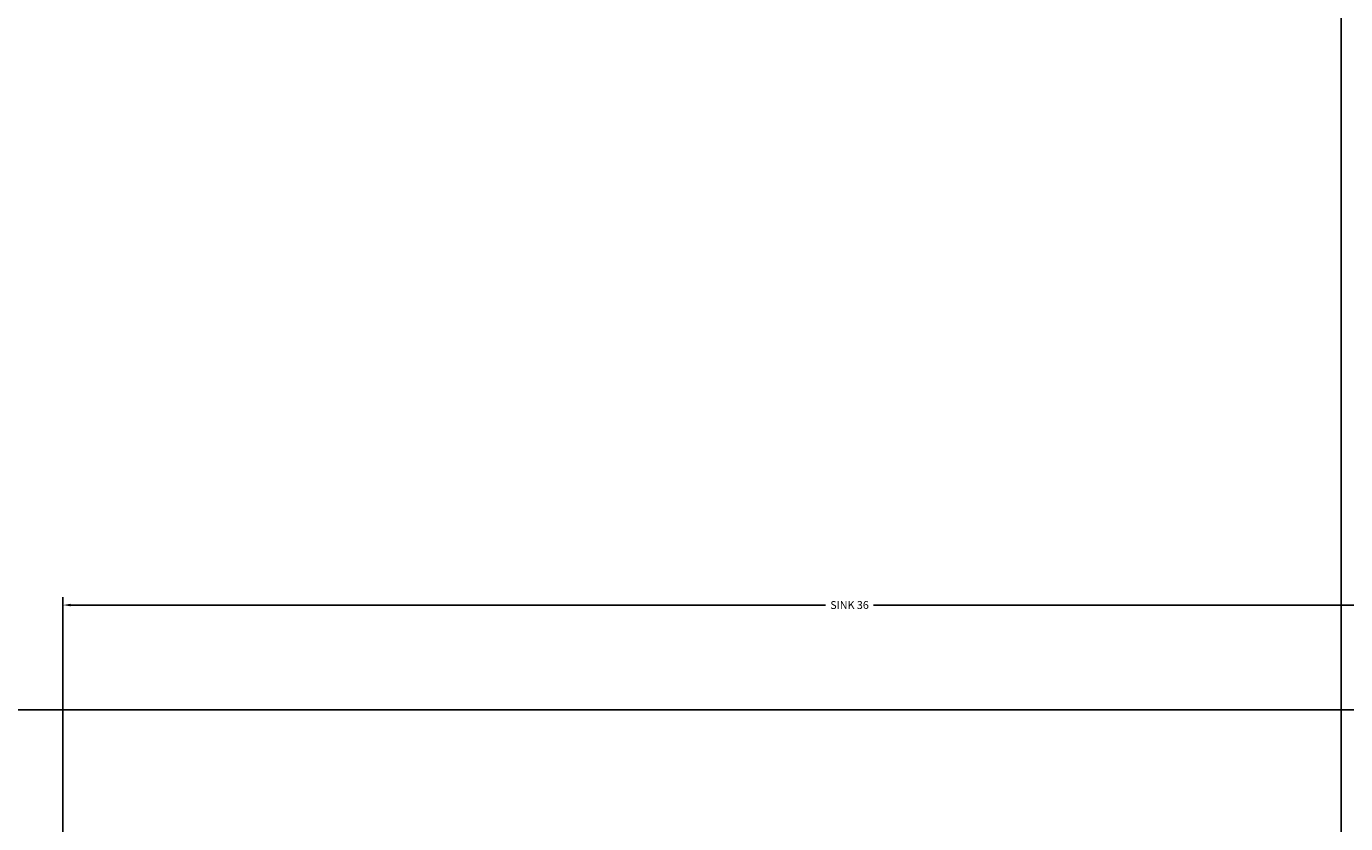
# Model space of a CAD drawing. Units: inches. Extents: x 2231 to 2461, y 2045 to 2455.
# Tile 20 of 95: x 2365 to 2395, y 2094 to 2112. Entities that reach past the tile are written whole.
import ezdxf

# ---------------------------------------------------------------- set-up
doc = ezdxf.new("R2010")
doc.units = ezdxf.units.IN
doc.layers.add('A-ANNO-DIMS', color=2, linetype='Continuous', lineweight=18)
doc.layers.add('A-FLOR-CASE', color=8, linetype='Continuous', lineweight=25)
doc.styles.get("Standard").update_dxf_attribs({"font": 'arial.ttf'})
doc.dimstyles.get("Standard").update_dxf_attribs({"dimtxt": 0.18, "dimasz": 0.18, "dimexe": 0.18, "dimexo": 0.0625, "dimgap": 0.09, "dimtad": 0, "dimtih": 1, "dimtoh": 1, "dimdec": 4, "dimzin": 0, "dimdsep": 46, "dimtxsty": 'Standard', "dimcen": 0.09, "dimadec": 0, "dimazin": 0, "dimtfac": 1, "dimtdec": 4, "dimtofl": 0, "dimtmove": 0, "dimatfit": 3, "dimfxl": 1, "dimtolj": 1, "dimtzin": 0, "dimarcsym": 0})

# ---------------------------------------------------------------- blocks, each defined once
blk = doc.blocks.new('*D29')
at = {"layer": 'A-ANNO-DIMS', "color": 0, "lineweight": -2, "transparency": 16777216}
for p, q in [((2365.54, 2093.895), (2365.54, 2099.413)), ((2401.54, 2093.895), (2401.54, 2099.413)), ((2365.72, 2099.233), (2382.993, 2099.233)), ((2401.36, 2099.233), (2384.087, 2099.233))]:
    blk.add_line(p, q, dxfattribs=at)
at = {"layer": 'A-ANNO-DIMS', "color": 0, "transparency": 16777216}
for points in [[(2365.72, 2099.263), (2365.72, 2099.203), (2365.54, 2099.233)], [(2401.36, 2099.263), (2401.36, 2099.203), (2401.54, 2099.233)]]:
    blk.add_solid(points, dxfattribs=at)
at = {"layer": 'Defpoints', "color": 0, "transparency": 16777216}
for p in [(2365.54, 2099.233), (2365.54, 2093.833), (2401.54, 2093.833)]:
    blk.add_point(p, dxfattribs=at)
at = {"layer": 'A-ANNO-DIMS', "color": 0, "transparency": 16777216, "insert": (2383.54, 2099.233), "char_height": 0.18, "attachment_point": 5}
blk.add_mtext('\\A1;SINK 36', dxfattribs=at)
blk = doc.blocks.new('*D66')
at = {"layer": 'A-ANNO-DIMS', "color": 0, "lineweight": -2, "transparency": 16777216}
for p, q in [((2348.189, 2096.895), (2348.189, 2454.645)), ((2348.369, 2454.465), (2378.167, 2454.465)), ((2408.614, 2454.465), (2378.815, 2454.465)), ((2408.794, 2096.895), (2408.794, 2454.645))]:
    blk.add_line(p, q, dxfattribs=at)
at = {"layer": 'A-ANNO-DIMS', "color": 0, "transparency": 16777216}
for points in [[(2348.369, 2454.495), (2348.369, 2454.435), (2348.189, 2454.465)], [(2408.614, 2454.495), (2408.614, 2454.435), (2408.794, 2454.465)]]:
    blk.add_solid(points, dxfattribs=at)
at = {"layer": 'Defpoints', "color": 0, "transparency": 16777216}
for p in [(2408.794, 2454.465), (2348.189, 2096.833), (2408.794, 2096.833)]:
    blk.add_point(p, dxfattribs=at)
at = {"layer": 'A-ANNO-DIMS', "color": 0, "transparency": 16777216, "insert": (2378.491, 2454.465), "char_height": 0.18, "attachment_point": 5}
blk.add_mtext('\\A1;60.6', dxfattribs=at)
blk = doc.blocks.new('*D69')
at = {"layer": 'A-ANNO-DIMS', "color": 0, "lineweight": -2, "transparency": 16777216}
for p, q in [((2340.667, 2189.285), (2340.667, 2044.803)), ((2394.794, 2186.77), (2394.794, 2044.803)), ((2340.847, 2044.983), (2367.337, 2044.983)), ((2394.614, 2044.983), (2368.124, 2044.983))]:
    blk.add_line(p, q, dxfattribs=at)
at = {"layer": 'A-ANNO-DIMS', "color": 0, "transparency": 16777216}
for points in [[(2340.847, 2045.013), (2340.847, 2044.953), (2340.667, 2044.983)], [(2394.614, 2045.013), (2394.614, 2044.953), (2394.794, 2044.983)]]:
    blk.add_solid(points, dxfattribs=at)
at = {"layer": 'Defpoints', "color": 0, "transparency": 16777216}
for p in [(2340.667, 2189.348), (2394.794, 2186.833), (2394.794, 2044.983)]:
    blk.add_point(p, dxfattribs=at)
at = {"layer": 'A-ANNO-DIMS', "color": 0, "transparency": 16777216, "insert": (2367.73, 2044.983), "char_height": 0.18, "attachment_point": 5}
blk.add_mtext('\\A1;54.13', dxfattribs=at)

msp = doc.modelspace()

# ---------------------------------------------------------------- linework, layer by layer
at = {"layer": 'A-FLOR-CASE'}
msp.add_line((2408.7935, 2096.8328), (2348.1888, 2096.8328), dxfattribs=at)

# ---------------------------------------------------------------- dimensions: what is measured, and where the dimension line sits
at = {"layer": 'A-ANNO-DIMS'}
for base, p1, p2, override, picture, middle in [((2408.7935, 2454.4653), (2348.1888, 2096.8328), (2408.7935, 2096.8328), {"dimdec": 1, "dimlfac": 1, "dimrnd": 0, "dimzin": 0, "dimdsep": 46, "dimlunit": 2}, '*D66', (2378.4912, 2454.4653)), ((2394.7935, 2044.9825), (2340.6673, 2189.3477), (2394.7935, 2186.8328), {"dimdec": 2, "dimlfac": 1, "dimrnd": 0, "dimzin": 0, "dimdsep": 46, "dimlunit": 2}, '*D69', (2367.7304, 2044.9825))]:
    dim = msp.add_linear_dim(base=base, p1=p1, p2=p2, dimstyle='Standard', override=override, dxfattribs=at)
    dim.commit()
    dim.dimension.update_dxf_attribs({"geometry": picture, "text_midpoint": middle})
dim = msp.add_linear_dim(base=(2365.54, 2099.2328), p1=(2401.54, 2093.8328), p2=(2365.54, 2093.8328), angle=180, text='SINK <>', dimstyle='Standard', override={"dimdec": 0, "dimlfac": 1, "dimrnd": 0, "dimzin": 0, "dimdsep": 46, "dimlunit": 2}, dxfattribs=at)
dim.commit()
dim.dimension.update_dxf_attribs({"geometry": '*D29', "text_midpoint": (2383.54, 2099.2328)})

doc.saveas('drawing.dxf')
